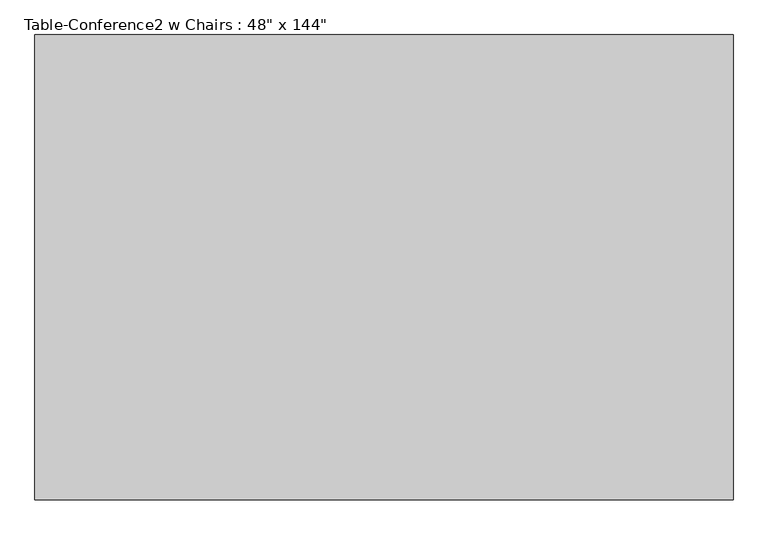
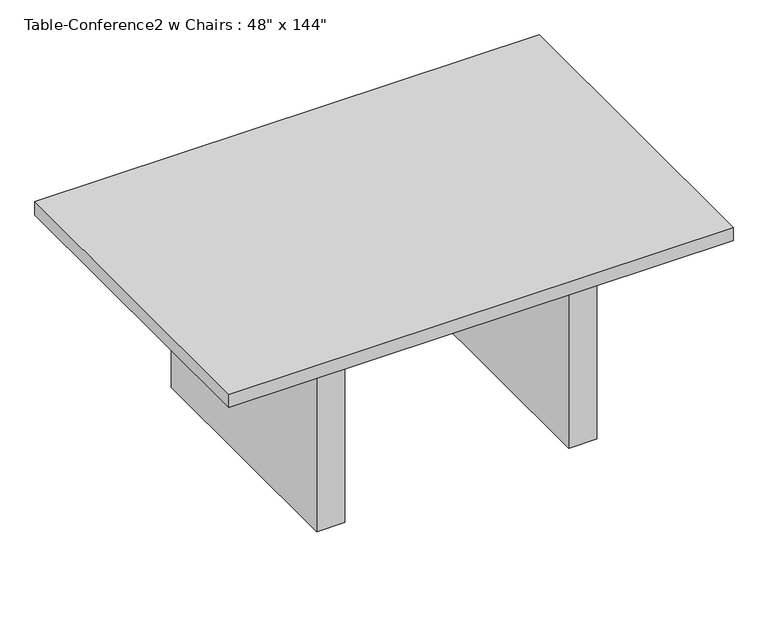
"""IFC4 building model written with IfcOpenShell, lengths in millimetres: furniture geometry."""

from ifc_helpers import new_model, si_unit, frame, origin, origin_with_axes, place, context, project, spatial, polyline, outline, extrude, source, transform, mapped, element, save


def furniture_0bcc43ae(model_context):
    return source(origin(), model_context, "Body", "SweptSolid", [
        extrude(outline(polyline([(914.4, -609.6), (-914.4, -609.6), (-914.4, 609.6), (914.4, 609.6), (914.4, -609.6)])), frame((0.0, 0.0, 711.2), z_axis=(0.0, 0.0, 1.0), x_axis=(1.0, 0.0, 0.0)), (0.0, 0.0, 1.0), 50.8),
        extrude(outline(polyline([(-406.4, -457.2), (-508.0, -457.2), (-508.0, 457.2), (-406.4, 457.2), (-406.4, -457.2)])), origin_with_axes(), (0.0, 0.0, 1.0), 711.2),
        extrude(outline(polyline([(508.0, -457.2), (406.4, -457.2), (406.4, 457.2), (508.0, 457.2), (508.0, -457.2)])), origin_with_axes(), (0.0, 0.0, 1.0), 711.2),
        extrude(outline(polyline([(406.4, 457.2), (406.4, 419.1), (-406.4, 419.1), (-406.4, 457.2), (406.4, 457.2)])), frame((0.0, 0.0, 609.6), z_axis=(0.0, 0.0, 1.0), x_axis=(1.0, 0.0, 0.0)), (0.0, 0.0, 1.0), 101.6),
        extrude(outline(polyline([(406.4, -457.2), (-406.4, -457.2), (-406.4, -419.1), (406.4, -419.1), (406.4, -457.2)])), frame((0.0, 0.0, 609.6), z_axis=(0.0, 0.0, 1.0), x_axis=(1.0, 0.0, 0.0)), (0.0, 0.0, 1.0), 101.6),
    ])


if __name__ == "__main__":
    model = new_model("IFC4")
    model_context = context("Model", 3, world=origin())
    ifc_project = project(units=[si_unit("LENGTHUNIT", "METRE", prefix="MILLI")], contexts=[model_context])
    site = spatial("IfcSite", under=ifc_project)
    building = spatial("IfcBuilding", under=site)
    placement = place(None, origin())
    furniture_shape = furniture_0bcc43ae(model_context)
    element("IfcFurniture", 1, ObjectType="Table-Conference2 w Chairs : 48\" x 144\"", at=placement, inside=building, context=model_context, shape_type="MappedRepresentation", body=[
        mapped(furniture_shape, transform((0.0, 0.0, 0.0), x_axis=(1.0, 0.0, 0.0), y_axis=(0.0, 1.0, 0.0), z_axis=(0.0, 0.0, 1.0))),
    ])
    save(model, "model.ifc")

# Revit data of these elements
# Type "Table-Conference2 w Chairs : 48\" x 144\""
#   Assembly Code = "E2020200"
#   Description = "Seating 12-14"
#   Height = 2' - 6"
#   Length = 6' - 0"
#   Width = 4' - 0"
#   Number Of Chairs One Side = 2
#   Number Of Chairs = 6
#   Material = Wood - Cherry
#   Default Elevation = 0
# Element 1 (IfcFurniture, "Table-Conference2 w Chairs : 48\" x 144\"")
#   Materials on its faces: "Wood - Cherry"
# Materials
#   "Wood - Cherry": colour RGB 151 75 0, transparency 0
